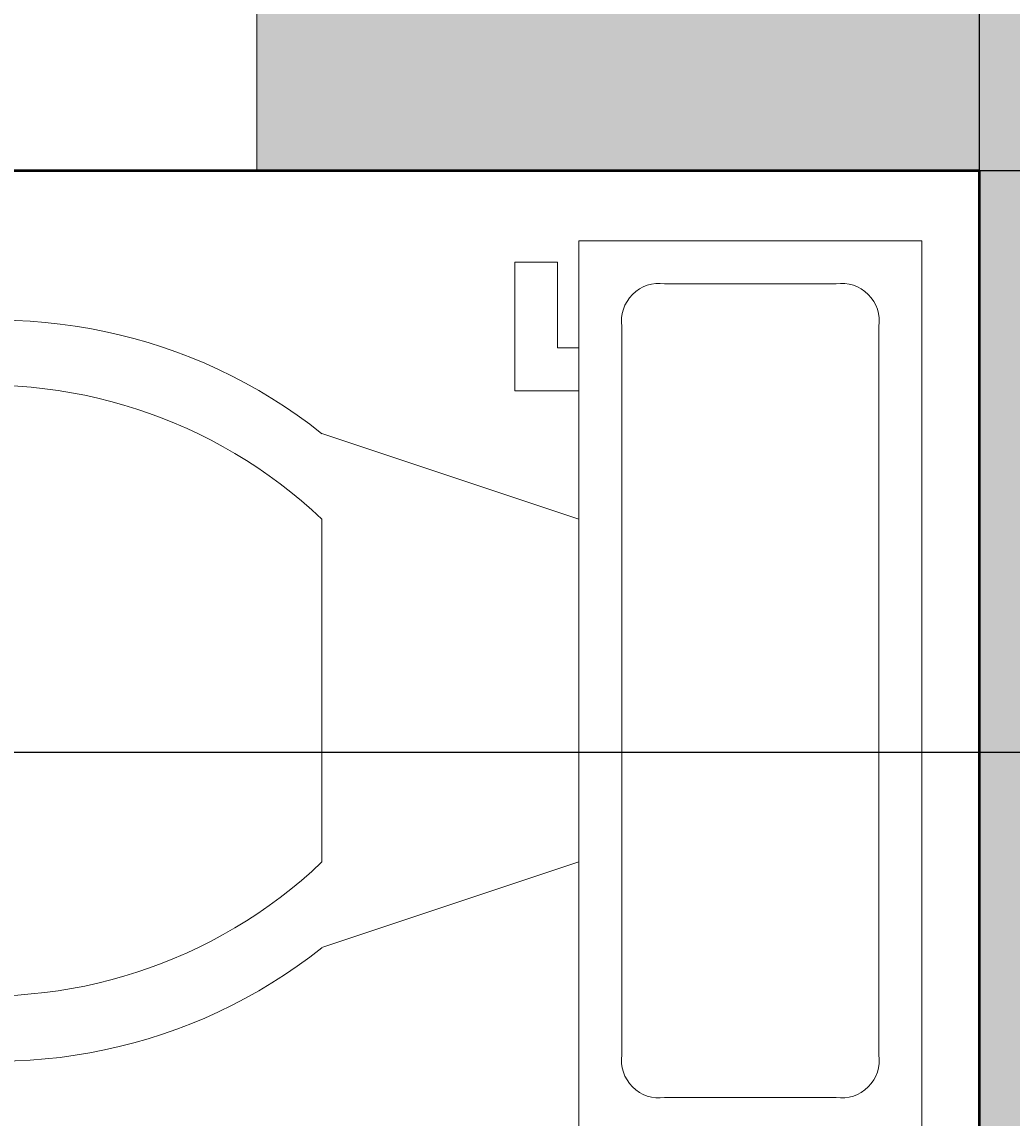
# Model space of a CAD drawing. Units: inches. Extents: x 2231 to 2461, y 2045 to 2455.
# Tile 92 of 95: x 2410 to 2434, y 2405 to 2430. Entities that reach past the tile are written whole.
import ezdxf

# ---------------------------------------------------------------- set-up
doc = ezdxf.new("R2010")
doc.units = ezdxf.units.IN
for name, color, linetype, lineweight in [('A-ANNO-DIMS', 2, 'Continuous', 18), ('A-FLOR-FIXT', 9, 'Continuous', 18), ('A-GLAZ', 4, 'Continuous', 18), ('A-WALL', 7, 'Continuous', 50)]:
    doc.layers.add(name, color=color, linetype=linetype, lineweight=lineweight)
doc.layers.add('A-WALL-PATT', color=18, linetype='Continuous', lineweight=13, true_color=0x000000)
doc.styles.get("Standard").update_dxf_attribs({"font": 'arial.ttf'})
doc.dimstyles.get("Standard").update_dxf_attribs({"dimtxt": 0.18, "dimasz": 0.18, "dimexe": 0.18, "dimexo": 0.0625, "dimgap": 0.09, "dimtad": 0, "dimtih": 1, "dimtoh": 1, "dimdec": 4, "dimzin": 0, "dimdsep": 46, "dimtxsty": 'Standard', "dimcen": 0.09, "dimadec": 0, "dimazin": 0, "dimtfac": 1, "dimtdec": 4, "dimtofl": 0, "dimtmove": 0, "dimatfit": 3, "dimfxl": 1, "dimtolj": 1, "dimtzin": 0, "dimarcsym": 0})

# ---------------------------------------------------------------- blocks, each defined once
blk = doc.blocks.new('Toilet - top')
for p, q in [((9.5, -6), (9.5, -2)), ((-8, -8.5), (-8, -8)), ((-7, -8), (-7, -9.5)), ((-4, -8), (-6, -14)), ((4, -8), (6, -14)), ((-10, -8.5), (-8, -8.5)), ((-10, -9.5), (-10, -8.5)), ((-7, -9.5), (-10, -9.5)), ((4, -14), (-4, -14))]:
    blk.add_line(p, q)
blk.add_lwpolyline([(10.5, -8), (10.5, 0), (-10.5, 0), (-10.5, -8)], close=True)
for points in [[(8.5, -1), (-8.5, -1)], [(-9.5, -2), (-9.5, -6)], [(-8.5, -7), (8.5, -7)]]:
    blk.add_lwpolyline(points)
for centre, radius, start, end in [((-8.625, -1.875), 0.884, 81.8699, 188.1301), ((8.625, -1.875), 0.884, 351.8699, 98.1301), ((-8.625, -6.125), 0.884, 171.8699, 278.1301), ((8.625, -6.125), 0.884, 261.8699, 8.1301), ((3.52, -21.58), 12.169, 141.4691, 247.9714), ((4.2, -21.817), 11.329, 136.3677, 238.9468), ((-3.519, -21.58), 12.169, 292.0284, 38.5307), ((-4.2, -21.817), 11.329, 301.053, 43.6321)]:
    blk.add_arc(centre, radius, start, end)
blk = doc.blocks.new('*D36')
at = {"layer": 'A-ANNO-DIMS', "color": 0, "lineweight": -2, "transparency": 16777216}
for p, q in [((2372.794, 2426.895), (2372.794, 2454.645)), ((2372.974, 2454.465), (2402.574, 2454.465)), ((2432.614, 2454.465), (2403.013, 2454.465)), ((2432.794, 2426.895), (2432.794, 2454.645))]:
    blk.add_line(p, q, dxfattribs=at)
at = {"layer": 'A-ANNO-DIMS', "color": 0, "transparency": 16777216}
for points in [[(2372.974, 2454.495), (2372.974, 2454.435), (2372.794, 2454.465)], [(2432.614, 2454.495), (2432.614, 2454.435), (2432.794, 2454.465)]]:
    blk.add_solid(points, dxfattribs=at)
at = {"layer": 'Defpoints', "color": 0, "transparency": 16777216}
for p in [(2432.794, 2454.465), (2372.794, 2426.833), (2432.794, 2426.833)]:
    blk.add_point(p, dxfattribs=at)
at = {"layer": 'A-ANNO-DIMS', "color": 0, "transparency": 16777216, "insert": (2402.794, 2454.465), "char_height": 0.18, "attachment_point": 5}
blk.add_mtext('\\A1;60', dxfattribs=at)
blk = doc.blocks.new('*D38')
at = {"layer": 'A-ANNO-DIMS', "color": 0, "lineweight": -2, "transparency": 16777216}
for p, q in [((2432.856, 2426.833), (2460.606, 2426.833)), ((2460.426, 2426.653), (2460.426, 2381.015)), ((2460.426, 2335.013), (2460.426, 2380.651)), ((2432.856, 2334.833), (2460.606, 2334.833))]:
    blk.add_line(p, q, dxfattribs=at)
at = {"layer": 'A-ANNO-DIMS', "color": 0, "transparency": 16777216}
for points in [[(2460.396, 2426.653), (2460.456, 2426.653), (2460.426, 2426.833)], [(2460.396, 2335.013), (2460.456, 2335.013), (2460.426, 2334.833)]]:
    blk.add_solid(points, dxfattribs=at)
at = {"layer": 'Defpoints', "color": 0, "transparency": 16777216}
for p in [(2432.794, 2426.833), (2460.426, 2426.833), (2432.794, 2334.833)]:
    blk.add_point(p, dxfattribs=at)
at = {"layer": 'A-ANNO-DIMS', "color": 0, "transparency": 16777216, "insert": (2460.426, 2380.833), "char_height": 0.18, "attachment_point": 5}
blk.add_mtext('\\A1;92', dxfattribs=at)
blk = doc.blocks.new('*D42')
at = {"layer": 'A-ANNO-DIMS', "color": 0, "lineweight": -2, "transparency": 16777216}
for p, q in [((2396.794, 2286.895), (2396.794, 2454.645)), ((2396.974, 2454.465), (2414.575, 2454.465)), ((2432.614, 2454.465), (2415.012, 2454.465)), ((2432.794, 2286.895), (2432.794, 2454.645))]:
    blk.add_line(p, q, dxfattribs=at)
at = {"layer": 'A-ANNO-DIMS', "color": 0, "transparency": 16777216}
for points in [[(2396.974, 2454.495), (2396.974, 2454.435), (2396.794, 2454.465)], [(2432.614, 2454.495), (2432.614, 2454.435), (2432.794, 2454.465)]]:
    blk.add_solid(points, dxfattribs=at)
at = {"layer": 'Defpoints', "color": 0, "transparency": 16777216}
for p in [(2432.794, 2454.465), (2396.794, 2286.833), (2432.794, 2286.833)]:
    blk.add_point(p, dxfattribs=at)
at = {"layer": 'A-ANNO-DIMS', "color": 0, "transparency": 16777216, "insert": (2414.794, 2454.465), "char_height": 0.18, "attachment_point": 5}
blk.add_mtext('\\A1;36', dxfattribs=at)
blk = doc.blocks.new('*D59')
at = {"layer": 'A-ANNO-DIMS', "color": 0, "lineweight": -2, "transparency": 16777216}
for p, q in [((2408.794, 2182.895), (2408.794, 2454.645)), ((2408.974, 2454.465), (2420.573, 2454.465)), ((2432.614, 2454.465), (2421.014, 2454.465)), ((2432.794, 2182.895), (2432.794, 2454.645))]:
    blk.add_line(p, q, dxfattribs=at)
at = {"layer": 'A-ANNO-DIMS', "color": 0, "transparency": 16777216}
for points in [[(2408.974, 2454.495), (2408.974, 2454.435), (2408.794, 2454.465)], [(2432.614, 2454.495), (2432.614, 2454.435), (2432.794, 2454.465)]]:
    blk.add_solid(points, dxfattribs=at)
at = {"layer": 'Defpoints', "color": 0, "transparency": 16777216}
for p in [(2432.794, 2454.465), (2408.794, 2182.833), (2432.794, 2182.833)]:
    blk.add_point(p, dxfattribs=at)
at = {"layer": 'A-ANNO-DIMS', "color": 0, "transparency": 16777216, "insert": (2420.794, 2454.465), "char_height": 0.18, "attachment_point": 5}
blk.add_mtext('\\A1;24', dxfattribs=at)
blk = doc.blocks.new('*D68')
at = {"layer": 'A-ANNO-DIMS', "color": 0, "lineweight": -2, "transparency": 16777216}
for p, q in [((2285.882, 2426.833), (2460.606, 2426.833)), ((2460.426, 2426.653), (2460.426, 2420.225)), ((2460.426, 2413.433), (2460.426, 2419.861)), ((2278.251, 2413.253), (2460.606, 2413.253))]:
    blk.add_line(p, q, dxfattribs=at)
at = {"layer": 'A-ANNO-DIMS', "color": 0, "transparency": 16777216}
for points in [[(2460.396, 2426.653), (2460.456, 2426.653), (2460.426, 2426.833)], [(2460.396, 2413.433), (2460.456, 2413.433), (2460.426, 2413.253)]]:
    blk.add_solid(points, dxfattribs=at)
at = {"layer": 'Defpoints', "color": 0, "transparency": 16777216}
for p in [(2285.82, 2426.833), (2460.426, 2426.833), (2278.188, 2413.253)]:
    blk.add_point(p, dxfattribs=at)
at = {"layer": 'A-ANNO-DIMS', "color": 0, "transparency": 16777216, "insert": (2460.426, 2420.043), "char_height": 0.18, "attachment_point": 5}
blk.add_mtext('\\A1;13.58', dxfattribs=at)

msp = doc.modelspace()

# ---------------------------------------------------------------- hatches: boundary and pattern name
at = {"layer": 'A-WALL-PATT'}
h = msp.add_hatch(color=256, dxfattribs=at)
h.dxf.hatch_style = 1
h.paths.add_polyline_path([(2441.7935, 2269.1535), (2432.7935, 2269.1535), (2432.7935, 2186.8328), (2396.7935, 2186.8328), (2396.7935, 2286.8328), (2394.7935, 2286.8328), (2394.7935, 2186.8328), (2334.7935, 2186.8328), (2334.7935, 2182.8328), (2432.7935, 2182.8328), (2432.7935, 2072.8328), (2416.6639, 2072.8328), (2416.6639, 2063.8328), (2441.7935, 2063.8328)])
h.paths.add_polyline_path([(2368.6639, 2072.8328), (2367.04, 2072.8328), (2330.7942, 2072.8328), (2330.7397, 2063.8328), (2368.6639, 2063.8328)])
h.paths.add_polyline_path([(2300.7392, 2068.3328), (2300.7392, 2072.8328), (2298.7935, 2072.8328), (2294.7935, 2072.8328), (2258.7935, 2072.8328), (2258.7935, 2120.8328), (2294.7935, 2120.8328), (2298.7935, 2120.8328), (2298.7935, 2128.8328), (2294.7935, 2128.8328), (2294.7935, 2124.8328), (2258.7935, 2124.8328), (2258.7935, 2182.8328), (2294.7935, 2182.8328), (2294.7935, 2174.8328), (2298.7935, 2174.8328), (2298.7935, 2182.8328), (2304.7935, 2182.8328), (2304.7935, 2186.8328), (2258.7935, 2186.8328), (2258.7935, 2221.999), (2249.7935, 2221.999), (2249.7935, 2063.8328), (2300.7392, 2063.8328)])
h.paths.add_polyline_path([(2391.9338, 2435.8328), (2333.82, 2435.8328), (2333.82, 2426.8328), (2368.7935, 2426.8328), (2368.7935, 2374.9508), (2368.7935, 2370.8328), (2372.3935, 2370.8328), (2372.7935, 2370.8328), (2372.7935, 2426.8328), (2391.9338, 2426.8328)])
h.paths.add_polyline_path([(2441.7935, 2435.8328), (2415.9338, 2435.8328), (2415.9338, 2426.8328), (2432.7935, 2426.8328), (2432.7935, 2334.8328), (2372.7935, 2334.8328), (2372.7935, 2346.8328), (2368.7935, 2346.8328), (2368.7935, 2306.8328), (2360.7935, 2306.8328), (2360.7935, 2302.8328), (2368.7935, 2302.8328), (2372.7935, 2302.8328), (2372.7935, 2330.8328), (2432.7935, 2330.8328), (2432.7935, 2317.1535), (2441.7935, 2317.1535)])
h.paths.add_polyline_path([(2285.82, 2435.8328), (2249.7935, 2435.8328), (2249.7935, 2269.999), (2258.7935, 2269.999), (2258.7935, 2302.8328), (2318.8168, 2302.8328), (2330.7935, 2302.8328), (2330.7935, 2306.8328), (2258.7935, 2306.8328), (2258.7935, 2426.8328), (2285.82, 2426.8328)])

# ---------------------------------------------------------------- linework, layer by layer
at = {"layer": 'A-GLAZ'}
msp.add_line((2415.9338, 2435.8328), (2415.9338, 2426.8328), dxfattribs=at)
at = {"layer": 'A-WALL'}
for p, q in [((2372.7935, 2426.8328), (2432.7935, 2426.8328)), ((2432.7935, 2426.8328), (2432.7935, 2334.8328))]:
    msp.add_line(p, q, dxfattribs=at)

# ---------------------------------------------------------------- block references
at = {"layer": 'A-FLOR-FIXT', "rotation": 270}
msp.add_blockref('Toilet - top', (2431.4505, 2414.6888), dxfattribs=at)

# ---------------------------------------------------------------- dimensions: what is measured, and where the dimension line sits
at = {"layer": 'A-ANNO-DIMS'}
for p1, p2, picture, middle in [((2372.7935, 2426.8328), (2432.7935, 2426.8328), '*D36', (2402.7935, 2454.4653)), ((2396.7935, 2286.8328), (2432.7935, 2286.8328), '*D42', (2414.7935, 2454.4653)), ((2408.7935, 2182.8328), (2432.7935, 2182.8328), '*D59', (2420.7935, 2454.4653))]:
    dim = msp.add_linear_dim(base=(2432.7935, 2454.4653), p1=p1, p2=p2, dimstyle='Standard', override={"dimdec": 0, "dimlfac": 1, "dimrnd": 0, "dimzin": 0, "dimdsep": 46, "dimlunit": 2}, dxfattribs=at)
    dim.commit()
    dim.dimension.update_dxf_attribs({"geometry": picture, "text_midpoint": middle})
for p1, p2, override, picture, middle in [((2278.1881, 2413.2534), (2285.82, 2426.8328), {"dimdec": 2, "dimlfac": 1, "dimrnd": 0, "dimzin": 0, "dimdsep": 46, "dimlunit": 2}, '*D68', (2460.426, 2420.0431)), ((2432.7935, 2334.8328), (2432.7935, 2426.8328), {"dimdec": 0, "dimlfac": 1, "dimrnd": 0, "dimzin": 0, "dimdsep": 46, "dimlunit": 2}, '*D38', (2460.426, 2380.8328))]:
    dim = msp.add_linear_dim(base=(2460.426, 2426.8328), p1=p1, p2=p2, angle=90, dimstyle='Standard', override=override, dxfattribs=at)
    dim.commit()
    dim.dimension.update_dxf_attribs({"geometry": picture, "text_midpoint": middle})

doc.saveas('drawing.dxf')
